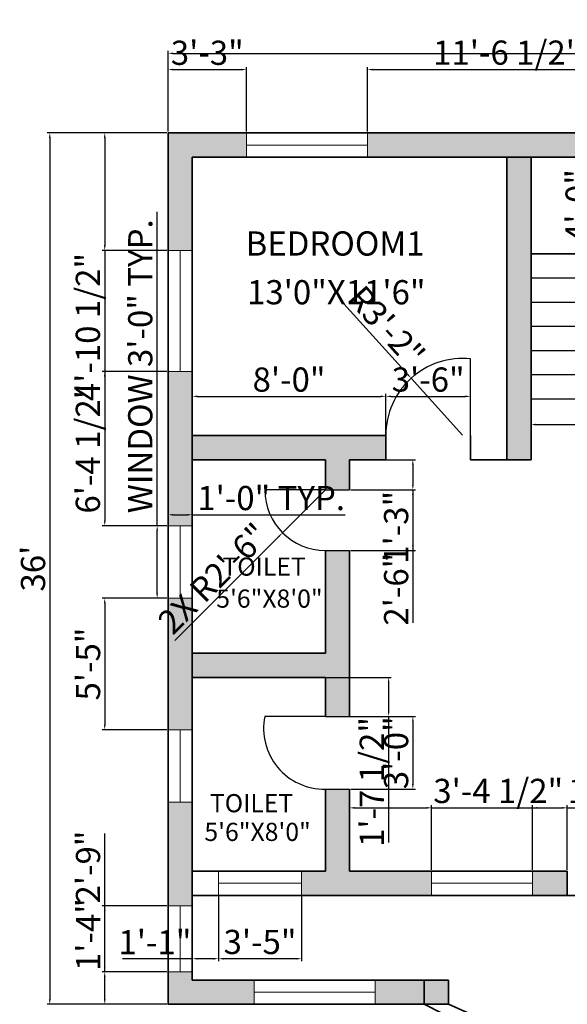
# Model space of a CAD drawing. Units: inches. Extents: x 1749 to 2426, y 1666 to 2412.
# Tile 2 of 3: x 1749 to 2021, y 1924 to 2412. Entities that reach past the tile are written whole.
import ezdxf

# ---------------------------------------------------------------- set-up
doc = ezdxf.new("R2010")
doc.units = ezdxf.units.IN
for name, color, linetype, lineweight in [('A-ANNO-DIMS', 2, 'Continuous', 18), ('A-AREA-IDEN', 4, 'Continuous', 18), ('A-DOOR', 6, 'Continuous', 25), ('A-FLOR-STRS', 7, 'Continuous', 25), ('A-GLAZ', 1, 'Continuous', 18), ('A-WALL', 2, 'Continuous', 35)]:
    doc.layers.add(name, color=color, linetype=linetype, lineweight=lineweight)
doc.layers.add('A-WALL-PATT', color=18, linetype='Continuous', lineweight=13, true_color=0x000000)
doc.styles.get("Standard").update_dxf_attribs({"font": 'arial.ttf'})
doc.dimstyles.new('ISO-25', dxfattribs={"dimtxt": 12, "dimasz": 2.5, "dimexe": 1.25, "dimexo": 0.625, "dimtad": 1, "dimdec": 0, "dimlunit": 3, "dimtxsty": 'Standard', "dimcen": 2.5, "dimadec": 0, "dimazin": 0, "dimtfac": 1, "dimtdec": 0, "dimtmove": 0, "dimatfit": 3, "dimfxl": 1, "dimarcsym": 0})

# ---------------------------------------------------------------- blocks, each defined once
blk = doc.blocks.new('*D1')
at = {"layer": 'A-ANNO-DIMS', "color": 0, "lineweight": -2, "transparency": 16777216}
for p, q in [((1822.59, 2356.85), (1822.59, 2396.9)), ((2374.59, 2356.85), (2374.59, 2396.9)), ((1825.09, 2395.65), (2372.09, 2395.65))]:
    blk.add_line(p, q, dxfattribs=at)
at = {"layer": 'A-ANNO-DIMS', "color": 0, "transparency": 16777216}
for points in [[(1825.09, 2396.07), (1825.09, 2395.23), (1822.59, 2395.65)], [(2372.09, 2396.07), (2372.09, 2395.23), (2374.59, 2395.65)]]:
    blk.add_solid(points, dxfattribs=at)
at = {"layer": 'Defpoints', "color": 0, "transparency": 16777216}
for p in [(2374.59, 2395.65), (1822.59, 2356.22), (2374.59, 2356.22)]:
    blk.add_point(p, dxfattribs=at)
at = {"layer": 'A-ANNO-DIMS', "color": 0, "transparency": 16777216, "insert": (2098.59, 2402.4), "char_height": 12, "attachment_point": 5}
blk.add_mtext("46'", dxfattribs=at)
blk = doc.blocks.new('*D2')
at = {"layer": 'A-ANNO-DIMS', "color": 0, "lineweight": -2, "transparency": 16777216}
for p, q in [((1821.97, 2356.22), (1762.68, 2356.22)), ((1763.93, 2353.72), (1763.93, 1926.72)), ((1821.97, 1924.22), (1762.68, 1924.22))]:
    blk.add_line(p, q, dxfattribs=at)
at = {"layer": 'A-ANNO-DIMS', "color": 0, "transparency": 16777216}
for points in [[(1763.52, 2353.72), (1764.35, 2353.72), (1763.93, 2356.22)], [(1763.52, 1926.72), (1764.35, 1926.72), (1763.93, 1924.22)]]:
    blk.add_solid(points, dxfattribs=at)
at = {"layer": 'Defpoints', "color": 0, "transparency": 16777216}
for p in [(1822.59, 2356.22), (1763.93, 1924.22), (1822.59, 1924.22)]:
    blk.add_point(p, dxfattribs=at)
at = {"layer": 'A-ANNO-DIMS', "color": 0, "transparency": 16777216, "insert": (1757.18, 2140.22), "char_height": 12, "attachment_point": 5, "rotation": 90}
blk.add_mtext("36'", dxfattribs=at)
blk = doc.blocks.new('WIN-60IN')
for p, q in [((12, 60), (0, 60)), ((6, 0), (6, 60)), ((6, 60), (12, 60)), ((0, 0), (12, 0))]:
    blk.add_line(p, q)
blk = doc.blocks.new('WIN-36IN')
for p, q in [((0, 36), (12, 36)), ((6, 36), (6, 0)), ((6, 0), (0, 0)), ((6, 0), (12, 0))]:
    blk.add_line(p, q)
blk = doc.blocks.new('WIN-50IN')
for p, q in [((0, 0), (0, 12)), ((50, 12), (50, 0)), ((50, 6), (0, 6)), ((0, 6), (0, 0))]:
    blk.add_line(p, q)
blk = doc.blocks.new('STAIR-FLIGHT-84IN')
for p, q in [((84, 72), (0, 72)), ((84, 60), (0, 60)), ((84, 48), (0, 48)), ((84, 36), (0, 36)), ((84, 24), (0, 24)), ((84, 12), (0, 12)), ((84, 0), (0, 0))]:
    blk.add_line(p, q)
blk = doc.blocks.new('*D9')
at = {"layer": 'A-ANNO-DIMS', "color": 0, "lineweight": -2, "transparency": 16777216}
for p, q in [((1817.19, 2161.49), (1817.19, 2317.09)), ((1821.97, 2161.49), (1815.94, 2161.49)), ((1817.19, 2127.99), (1817.19, 2158.99)), ((1821.97, 2125.49), (1815.94, 2125.49))]:
    blk.add_line(p, q, dxfattribs=at)
at = {"layer": 'A-ANNO-DIMS', "color": 0, "transparency": 16777216}
for points in [[(1816.77, 2158.99), (1817.61, 2158.99), (1817.19, 2161.49)], [(1816.77, 2127.99), (1817.61, 2127.99), (1817.19, 2125.49)]]:
    blk.add_solid(points, dxfattribs=at)
at = {"layer": 'Defpoints', "color": 0, "transparency": 16777216}
for p in [(1817.19, 2161.49), (1822.59, 2161.49), (1822.59, 2125.49)]:
    blk.add_point(p, dxfattribs=at)
at = {"layer": 'A-ANNO-DIMS', "color": 0, "transparency": 16777216, "insert": (1810.35, 2240.54), "char_height": 12, "attachment_point": 5, "rotation": 90}
blk.add_mtext('WINDOW 3\'-0" TYP.', dxfattribs=at)
blk = doc.blocks.new('*D10')
at = {"layer": 'A-ANNO-DIMS', "color": 0, "lineweight": -2, "transparency": 16777216}
for p, q in [((1822.59, 2162.12), (1822.59, 2168.14)), ((1834.59, 2162.12), (1834.59, 2168.14)), ((1825.09, 2166.89), (1832.09, 2166.89)), ((1834.59, 2166.89), (1910.36, 2166.89))]:
    blk.add_line(p, q, dxfattribs=at)
at = {"layer": 'A-ANNO-DIMS', "color": 0, "transparency": 16777216}
for points in [[(1825.09, 2167.31), (1825.09, 2166.48), (1822.59, 2166.89)], [(1832.09, 2167.31), (1832.09, 2166.48), (1834.59, 2166.89)]]:
    blk.add_solid(points, dxfattribs=at)
at = {"layer": 'Defpoints', "color": 0, "transparency": 16777216}
for p in [(1834.59, 2166.89), (1822.59, 2161.49), (1834.59, 2161.49)]:
    blk.add_point(p, dxfattribs=at)
at = {"layer": 'A-ANNO-DIMS', "color": 0, "transparency": 16777216, "insert": (1873.72, 2173.65), "char_height": 12, "attachment_point": 5}
blk.add_mtext('1\'-0" TYP.', dxfattribs=at)
blk = doc.blocks.new('*D13')
at = {"layer": 'A-ANNO-DIMS', "color": 0, "lineweight": -2, "transparency": 16777216}
for p, q in [((2002.59, 2223.6), (2002.59, 2210.37)), ((2086.59, 2223.6), (2086.59, 2210.37)), ((2005.09, 2211.62), (2084.09, 2211.62)), ((2086.59, 2211.62), (2281.72, 2211.62))]:
    blk.add_line(p, q, dxfattribs=at)
at = {"layer": 'A-ANNO-DIMS', "color": 0, "transparency": 16777216}
for points in [[(2005.09, 2212.04), (2005.09, 2211.2), (2002.59, 2211.62)], [(2084.09, 2212.04), (2084.09, 2211.2), (2086.59, 2211.62)]]:
    blk.add_solid(points, dxfattribs=at)
at = {"layer": 'Defpoints', "color": 0, "transparency": 16777216}
for p in [(2002.59, 2224.22), (2086.59, 2224.22), (2086.59, 2211.62)]:
    blk.add_point(p, dxfattribs=at)
at = {"layer": 'A-ANNO-DIMS', "color": 0, "transparency": 16777216, "insert": (2185.41, 2218.45), "char_height": 12, "attachment_point": 5}
blk.add_mtext('STAIR FLIGHT 7\'-0" TYP.', dxfattribs=at)
blk = doc.blocks.new('*D15')
at = {"layer": 'A-ANNO-DIMS', "color": 0, "lineweight": -2, "transparency": 16777216}
for p, q in [((1822.59, 2356.85), (1822.59, 2388.87)), ((1825.09, 2387.62), (1858.99, 2387.62)), ((1861.49, 2356.85), (1861.49, 2388.87))]:
    blk.add_line(p, q, dxfattribs=at)
at = {"layer": 'A-ANNO-DIMS', "color": 0, "transparency": 16777216}
for points in [[(1825.09, 2388.04), (1825.09, 2387.2), (1822.59, 2387.62)], [(1858.99, 2388.04), (1858.99, 2387.2), (1861.49, 2387.62)]]:
    blk.add_solid(points, dxfattribs=at)
at = {"layer": 'Defpoints', "color": 0, "transparency": 16777216}
for p in [(1861.49, 2387.62), (1822.59, 2356.22), (1861.49, 2356.22)]:
    blk.add_point(p, dxfattribs=at)
at = {"layer": 'A-ANNO-DIMS', "color": 0, "transparency": 16777216, "insert": (1842.04, 2394.38), "char_height": 12, "attachment_point": 5}
blk.add_mtext('3\'-3"', dxfattribs=at)
blk = doc.blocks.new('*D16')
at = {"layer": 'A-ANNO-DIMS', "color": 0, "lineweight": -2, "transparency": 16777216}
for p, q in [((1921.49, 2356.85), (1921.49, 2388.87)), ((1923.99, 2387.62), (2057.63, 2387.62)), ((2060.13, 2356.85), (2060.13, 2388.87))]:
    blk.add_line(p, q, dxfattribs=at)
at = {"layer": 'A-ANNO-DIMS', "color": 0, "transparency": 16777216}
for points in [[(1923.99, 2388.04), (1923.99, 2387.2), (1921.49, 2387.62)], [(2057.63, 2388.04), (2057.63, 2387.2), (2060.13, 2387.62)]]:
    blk.add_solid(points, dxfattribs=at)
at = {"layer": 'Defpoints', "color": 0, "transparency": 16777216}
for p in [(2060.13, 2387.62), (1921.49, 2356.22), (2060.13, 2356.22)]:
    blk.add_point(p, dxfattribs=at)
at = {"layer": 'A-ANNO-DIMS', "color": 0, "transparency": 16777216, "insert": (1990.81, 2394.45), "char_height": 12, "attachment_point": 5}
blk.add_mtext('11\'-6 1/2"', dxfattribs=at)
blk = doc.blocks.new('*D19')
at = {"layer": 'A-ANNO-DIMS', "color": 0, "lineweight": -2, "transparency": 16777216}
for p, q in [((1821.97, 2356.22), (1789.94, 2356.22)), ((1791.19, 2353.72), (1791.19, 2300.45)), ((1821.97, 2297.95), (1789.94, 2297.95)), ((1791.19, 2297.95), (1791.19, 2224.53))]:
    blk.add_line(p, q, dxfattribs=at)
at = {"layer": 'A-ANNO-DIMS', "color": 0, "transparency": 16777216}
for points in [[(1790.77, 2353.72), (1791.61, 2353.72), (1791.19, 2356.22)], [(1790.77, 2300.45), (1791.61, 2300.45), (1791.19, 2297.95)]]:
    blk.add_solid(points, dxfattribs=at)
at = {"layer": 'Defpoints', "color": 0, "transparency": 16777216}
for p in [(1822.59, 2356.22), (1791.19, 2297.95), (1822.59, 2297.95)]:
    blk.add_point(p, dxfattribs=at)
at = {"layer": 'A-ANNO-DIMS', "color": 0, "transparency": 16777216, "insert": (1784.36, 2259.99), "char_height": 12, "attachment_point": 5, "rotation": 90}
blk.add_mtext('4\'-10 1/2"', dxfattribs=at)
blk = doc.blocks.new('*D20')
at = {"layer": 'A-ANNO-DIMS', "color": 0, "lineweight": -2, "transparency": 16777216}
for p, q in [((1821.97, 2237.95), (1789.94, 2237.95)), ((1791.19, 2235.45), (1791.19, 2163.99)), ((1821.97, 2161.49), (1789.94, 2161.49))]:
    blk.add_line(p, q, dxfattribs=at)
at = {"layer": 'A-ANNO-DIMS', "color": 0, "transparency": 16777216}
for points in [[(1790.77, 2235.45), (1791.61, 2235.45), (1791.19, 2237.95)], [(1790.77, 2163.99), (1791.61, 2163.99), (1791.19, 2161.49)]]:
    blk.add_solid(points, dxfattribs=at)
at = {"layer": 'Defpoints', "color": 0, "transparency": 16777216}
for p in [(1822.59, 2237.95), (1791.19, 2161.49), (1822.59, 2161.49)]:
    blk.add_point(p, dxfattribs=at)
at = {"layer": 'A-ANNO-DIMS', "color": 0, "transparency": 16777216, "insert": (1784.36, 2199.72), "char_height": 12, "attachment_point": 5, "rotation": 90}
blk.add_mtext('6\'-4 1/2"', dxfattribs=at)
blk = doc.blocks.new('*D21')
at = {"layer": 'A-ANNO-DIMS', "color": 0, "lineweight": -2, "transparency": 16777216}
for p, q in [((1821.97, 2125.49), (1789.94, 2125.49)), ((1791.19, 2122.99), (1791.19, 2062.85)), ((1821.97, 2060.35), (1789.94, 2060.35))]:
    blk.add_line(p, q, dxfattribs=at)
at = {"layer": 'A-ANNO-DIMS', "color": 0, "transparency": 16777216}
for points in [[(1790.77, 2122.99), (1791.61, 2122.99), (1791.19, 2125.49)], [(1790.77, 2062.85), (1791.61, 2062.85), (1791.19, 2060.35)]]:
    blk.add_solid(points, dxfattribs=at)
at = {"layer": 'Defpoints', "color": 0, "transparency": 16777216}
for p in [(1822.59, 2125.49), (1791.19, 2060.35), (1822.59, 2060.35)]:
    blk.add_point(p, dxfattribs=at)
at = {"layer": 'A-ANNO-DIMS', "color": 0, "transparency": 16777216, "insert": (1784.46, 2092.92), "char_height": 12, "attachment_point": 5, "rotation": 90}
blk.add_mtext('5\'-5"', dxfattribs=at)
blk = doc.blocks.new('*D29')
at = {"layer": 'A-ANNO-DIMS', "color": 0, "lineweight": -2, "transparency": 16777216}
for p, q in [((1834.59, 2194.85), (1834.59, 2226.87)), ((1930.59, 2194.85), (1930.59, 2226.87)), ((1837.09, 2225.62), (1928.09, 2225.62))]:
    blk.add_line(p, q, dxfattribs=at)
at = {"layer": 'A-ANNO-DIMS', "color": 0, "transparency": 16777216}
for points in [[(1837.09, 2226.04), (1837.09, 2225.2), (1834.59, 2225.62)], [(1928.09, 2226.04), (1928.09, 2225.2), (1930.59, 2225.62)]]:
    blk.add_solid(points, dxfattribs=at)
at = {"layer": 'Defpoints', "color": 0, "transparency": 16777216}
for p in [(1930.59, 2225.62), (1834.59, 2194.22), (1930.59, 2194.22)]:
    blk.add_point(p, dxfattribs=at)
at = {"layer": 'A-ANNO-DIMS', "color": 0, "transparency": 16777216, "insert": (1882.59, 2232.37), "char_height": 12, "attachment_point": 5}
blk.add_mtext('8\'-0"', dxfattribs=at)
blk = doc.blocks.new('*D30')
at = {"layer": 'A-ANNO-DIMS', "color": 0, "lineweight": -2, "transparency": 16777216}
for p, q in [((1930.59, 2194.85), (1930.59, 2226.87)), ((1972.59, 2194.85), (1972.59, 2226.87)), ((1933.09, 2225.62), (1970.09, 2225.62))]:
    blk.add_line(p, q, dxfattribs=at)
at = {"layer": 'A-ANNO-DIMS', "color": 0, "transparency": 16777216}
for points in [[(1933.09, 2226.04), (1933.09, 2225.2), (1930.59, 2225.62)], [(1970.09, 2226.04), (1970.09, 2225.2), (1972.59, 2225.62)]]:
    blk.add_solid(points, dxfattribs=at)
at = {"layer": 'Defpoints', "color": 0, "transparency": 16777216}
for p in [(1972.59, 2225.62), (1930.59, 2194.22), (1972.59, 2194.22)]:
    blk.add_point(p, dxfattribs=at)
at = {"layer": 'A-ANNO-DIMS', "color": 0, "transparency": 16777216, "insert": (1951.59, 2232.38), "char_height": 12, "attachment_point": 5}
blk.add_mtext('3\'-6"', dxfattribs=at)
blk = doc.blocks.new('*D33')
at = {"layer": 'A-ANNO-DIMS', "color": 0, "lineweight": -2, "transparency": 16777216}
for p, q in [((2003.22, 2344.22), (2035.24, 2344.22)), ((2033.99, 2341.72), (2033.99, 2298.72)), ((2003.22, 2296.22), (2035.24, 2296.22))]:
    blk.add_line(p, q, dxfattribs=at)
at = {"layer": 'A-ANNO-DIMS', "color": 0, "transparency": 16777216}
for points in [[(2033.57, 2341.72), (2034.41, 2341.72), (2033.99, 2344.22)], [(2033.57, 2298.72), (2034.41, 2298.72), (2033.99, 2296.22)]]:
    blk.add_solid(points, dxfattribs=at)
at = {"layer": 'Defpoints', "color": 0, "transparency": 16777216}
for p in [(2002.59, 2344.22), (2002.59, 2296.22), (2033.99, 2296.22)]:
    blk.add_point(p, dxfattribs=at)
at = {"layer": 'A-ANNO-DIMS', "color": 0, "transparency": 16777216, "insert": (2027.24, 2320.22), "char_height": 12, "attachment_point": 5, "rotation": 90}
blk.add_mtext('4\'-0"', dxfattribs=at)
blk = doc.blocks.new('*D40')
at = {"layer": 'A-ANNO-DIMS', "color": 0, "lineweight": -2, "transparency": 16777216}
for p, q in [((1791.19, 1973.11), (1791.19, 2008.96)), ((1821.97, 1973.11), (1789.94, 1973.11)), ((1791.19, 1942.77), (1791.19, 1970.61)), ((1821.97, 1940.27), (1789.94, 1940.27))]:
    blk.add_line(p, q, dxfattribs=at)
at = {"layer": 'A-ANNO-DIMS', "color": 0, "transparency": 16777216}
for points in [[(1790.77, 1970.61), (1791.61, 1970.61), (1791.19, 1973.11)], [(1790.77, 1942.77), (1791.61, 1942.77), (1791.19, 1940.27)]]:
    blk.add_solid(points, dxfattribs=at)
at = {"layer": 'Defpoints', "color": 0, "transparency": 16777216}
for p in [(1791.19, 1973.11), (1822.59, 1973.11), (1822.59, 1940.27)]:
    blk.add_point(p, dxfattribs=at)
at = {"layer": 'A-ANNO-DIMS', "color": 0, "transparency": 16777216, "insert": (1784.44, 1992.28), "char_height": 12, "attachment_point": 5, "rotation": 90}
blk.add_mtext('2\'-9"', dxfattribs=at)
blk = doc.blocks.new('*D41')
at = {"layer": 'A-ANNO-DIMS', "color": 0, "lineweight": -2, "transparency": 16777216}
for p, q in [((1791.19, 1940.27), (1791.19, 1974.79)), ((1821.97, 1940.27), (1789.94, 1940.27)), ((1791.19, 1926.72), (1791.19, 1937.77)), ((1821.97, 1924.22), (1789.94, 1924.22))]:
    blk.add_line(p, q, dxfattribs=at)
at = {"layer": 'A-ANNO-DIMS', "color": 0, "transparency": 16777216}
for points in [[(1790.77, 1937.77), (1791.61, 1937.77), (1791.19, 1940.27)], [(1790.77, 1926.72), (1791.61, 1926.72), (1791.19, 1924.22)]]:
    blk.add_solid(points, dxfattribs=at)
at = {"layer": 'Defpoints', "color": 0, "transparency": 16777216}
for p in [(1791.19, 1940.27), (1822.59, 1940.27), (1822.59, 1924.22)]:
    blk.add_point(p, dxfattribs=at)
at = {"layer": 'A-ANNO-DIMS', "color": 0, "transparency": 16777216, "insert": (1784.54, 1958.78), "char_height": 12, "attachment_point": 5, "rotation": 90}
blk.add_mtext('1\'-4"', dxfattribs=at)
blk = doc.blocks.new('*D46')
at = {"layer": 'A-ANNO-DIMS', "color": 0, "lineweight": -2, "transparency": 16777216}
for p, q in [((1847.61, 1977.6), (1847.61, 1945.57)), ((1888.8, 1977.6), (1888.8, 1945.57)), ((1886.3, 1946.82), (1850.11, 1946.82))]:
    blk.add_line(p, q, dxfattribs=at)
at = {"layer": 'A-ANNO-DIMS', "color": 0, "transparency": 16777216}
for points in [[(1850.11, 1947.24), (1850.11, 1946.4), (1847.61, 1946.82)], [(1886.3, 1947.24), (1886.3, 1946.4), (1888.8, 1946.82)]]:
    blk.add_solid(points, dxfattribs=at)
at = {"layer": 'Defpoints', "color": 0, "transparency": 16777216}
for p in [(1847.61, 1978.22), (1888.8, 1978.22), (1847.61, 1946.82)]:
    blk.add_point(p, dxfattribs=at)
at = {"layer": 'A-ANNO-DIMS', "color": 0, "transparency": 16777216, "insert": (1868.2, 1953.58), "char_height": 12, "attachment_point": 5}
blk.add_mtext('3\'-5"', dxfattribs=at)
blk = doc.blocks.new('*D47')
at = {"layer": 'A-ANNO-DIMS', "color": 0, "lineweight": -2, "transparency": 16777216}
for p, q in [((1834.59, 1977.6), (1834.59, 1945.57)), ((1847.61, 1977.6), (1847.61, 1945.57)), ((1834.59, 1946.82), (1800.07, 1946.82)), ((1845.11, 1946.82), (1837.09, 1946.82))]:
    blk.add_line(p, q, dxfattribs=at)
at = {"layer": 'A-ANNO-DIMS', "color": 0, "transparency": 16777216}
for points in [[(1837.09, 1947.24), (1837.09, 1946.4), (1834.59, 1946.82)], [(1845.11, 1947.24), (1845.11, 1946.4), (1847.61, 1946.82)]]:
    blk.add_solid(points, dxfattribs=at)
at = {"layer": 'Defpoints', "color": 0, "transparency": 16777216}
for p in [(1834.59, 1978.22), (1847.61, 1978.22), (1834.59, 1946.82)]:
    blk.add_point(p, dxfattribs=at)
at = {"layer": 'A-ANNO-DIMS', "color": 0, "transparency": 16777216, "insert": (1816.08, 1953.47), "char_height": 12, "attachment_point": 5}
blk.add_mtext('1\'-1"', dxfattribs=at)
blk = doc.blocks.new('*D48')
at = {"layer": 'A-ANNO-DIMS', "color": 0, "lineweight": -2, "transparency": 16777216}
for p, q in [((1912.59, 1990.85), (1912.59, 2022.87)), ((1915.09, 2021.62), (1950.79, 2021.62)), ((1953.29, 1990.85), (1953.29, 2022.87)), ((1953.29, 2021.62), (2016.89, 2021.62))]:
    blk.add_line(p, q, dxfattribs=at)
at = {"layer": 'A-ANNO-DIMS', "color": 0, "transparency": 16777216}
for points in [[(1915.09, 2022.04), (1915.09, 2021.2), (1912.59, 2021.62)], [(1950.79, 2022.04), (1950.79, 2021.2), (1953.29, 2021.62)]]:
    blk.add_solid(points, dxfattribs=at)
at = {"layer": 'Defpoints', "color": 0, "transparency": 16777216}
for p in [(1953.29, 2021.62), (1912.59, 1990.22), (1953.29, 1990.22)]:
    blk.add_point(p, dxfattribs=at)
at = {"layer": 'A-ANNO-DIMS', "color": 0, "transparency": 16777216, "insert": (1986.34, 2028.45), "char_height": 12, "attachment_point": 5}
blk.add_mtext('3\'-4 1/2"', dxfattribs=at)
blk = doc.blocks.new('*D49')
at = {"layer": 'A-ANNO-DIMS', "color": 0, "lineweight": -2, "transparency": 16777216}
for p, q in [((2003.29, 1990.85), (2003.29, 2022.87)), ((2005.79, 2021.62), (2018.09, 2021.62)), ((2020.59, 1990.85), (2020.59, 2022.87)), ((2020.59, 2021.62), (2083.07, 2021.62))]:
    blk.add_line(p, q, dxfattribs=at)
at = {"layer": 'A-ANNO-DIMS', "color": 0, "transparency": 16777216}
for points in [[(2005.79, 2022.04), (2005.79, 2021.2), (2003.29, 2021.62)], [(2018.09, 2022.04), (2018.09, 2021.2), (2020.59, 2021.62)]]:
    blk.add_solid(points, dxfattribs=at)
at = {"layer": 'Defpoints', "color": 0, "transparency": 16777216}
for p in [(2020.59, 2021.62), (2003.29, 1990.22), (2020.59, 1990.22)]:
    blk.add_point(p, dxfattribs=at)
at = {"layer": 'A-ANNO-DIMS', "color": 0, "transparency": 16777216, "insert": (2053.08, 2028.45), "char_height": 12, "attachment_point": 5}
blk.add_mtext('1\'-5 1/2"', dxfattribs=at)
blk = doc.blocks.new('*D52')
at = {"layer": 'A-ANNO-DIMS', "color": 0, "lineweight": -2, "transparency": 16777216}
for p, q in [((1913.22, 2194.22), (1945.24, 2194.22)), ((1943.99, 2191.72), (1943.99, 2181.72)), ((1913.22, 2179.22), (1945.24, 2179.22)), ((1943.99, 2179.22), (1943.99, 2144.7))]:
    blk.add_line(p, q, dxfattribs=at)
at = {"layer": 'A-ANNO-DIMS', "color": 0, "transparency": 16777216}
for points in [[(1943.57, 2191.72), (1944.41, 2191.72), (1943.99, 2194.22)], [(1943.57, 2181.72), (1944.41, 2181.72), (1943.99, 2179.22)]]:
    blk.add_solid(points, dxfattribs=at)
at = {"layer": 'Defpoints', "color": 0, "transparency": 16777216}
for p in [(1912.59, 2194.22), (1912.59, 2179.22), (1943.99, 2179.22)]:
    blk.add_point(p, dxfattribs=at)
at = {"layer": 'A-ANNO-DIMS', "color": 0, "transparency": 16777216, "insert": (1937.24, 2160.71), "char_height": 12, "attachment_point": 5, "rotation": 90}
blk.add_mtext('1\'-3"', dxfattribs=at)
blk = doc.blocks.new('*D53')
at = {"layer": 'A-ANNO-DIMS', "color": 0, "lineweight": -2, "transparency": 16777216}
for p, q in [((1913.22, 2179.22), (1945.24, 2179.22)), ((1943.99, 2176.72), (1943.99, 2151.72)), ((1913.22, 2149.22), (1945.24, 2149.22)), ((1943.99, 2149.22), (1943.99, 2113.37))]:
    blk.add_line(p, q, dxfattribs=at)
at = {"layer": 'A-ANNO-DIMS', "color": 0, "transparency": 16777216}
for points in [[(1943.57, 2176.72), (1944.41, 2176.72), (1943.99, 2179.22)], [(1943.57, 2151.72), (1944.41, 2151.72), (1943.99, 2149.22)]]:
    blk.add_solid(points, dxfattribs=at)
at = {"layer": 'Defpoints', "color": 0, "transparency": 16777216}
for p in [(1912.59, 2179.22), (1912.59, 2149.22), (1943.99, 2149.22)]:
    blk.add_point(p, dxfattribs=at)
at = {"layer": 'A-ANNO-DIMS', "color": 0, "transparency": 16777216, "insert": (1937.24, 2130.04), "char_height": 12, "attachment_point": 5, "rotation": 90}
blk.add_mtext('2\'-6"', dxfattribs=at)
blk = doc.blocks.new('*D54')
at = {"layer": 'A-ANNO-DIMS', "color": 0, "lineweight": -2, "transparency": 16777216}
for p, q in [((1901.22, 2086.22), (1933.24, 2086.22)), ((1931.99, 2083.72), (1931.99, 2069.44)), ((1901.22, 2066.94), (1933.24, 2066.94)), ((1931.99, 2066.94), (1931.99, 2004.46))]:
    blk.add_line(p, q, dxfattribs=at)
at = {"layer": 'A-ANNO-DIMS', "color": 0, "transparency": 16777216}
for points in [[(1931.57, 2083.72), (1932.41, 2083.72), (1931.99, 2086.22)], [(1931.57, 2069.44), (1932.41, 2069.44), (1931.99, 2066.94)]]:
    blk.add_solid(points, dxfattribs=at)
at = {"layer": 'Defpoints', "color": 0, "transparency": 16777216}
for p in [(1900.59, 2086.22), (1900.59, 2066.94), (1931.99, 2066.94)]:
    blk.add_point(p, dxfattribs=at)
at = {"layer": 'A-ANNO-DIMS', "color": 0, "transparency": 16777216, "insert": (1925.16, 2034.45), "char_height": 12, "attachment_point": 5, "rotation": 90}
blk.add_mtext('1\'-7 1/2"', dxfattribs=at)
blk = doc.blocks.new('*D55')
at = {"layer": 'A-ANNO-DIMS', "color": 0, "lineweight": -2, "transparency": 16777216}
for p, q in [((1913.22, 2066.94), (1945.24, 2066.94)), ((1943.99, 2064.44), (1943.99, 2033.44)), ((1913.22, 2030.94), (1945.24, 2030.94))]:
    blk.add_line(p, q, dxfattribs=at)
at = {"layer": 'A-ANNO-DIMS', "color": 0, "transparency": 16777216}
for points in [[(1943.57, 2064.44), (1944.41, 2064.44), (1943.99, 2066.94)], [(1943.57, 2033.44), (1944.41, 2033.44), (1943.99, 2030.94)]]:
    blk.add_solid(points, dxfattribs=at)
at = {"layer": 'Defpoints', "color": 0, "transparency": 16777216}
for p in [(1912.59, 2066.94), (1912.59, 2030.94), (1943.99, 2030.94)]:
    blk.add_point(p, dxfattribs=at)
at = {"layer": 'A-ANNO-DIMS', "color": 0, "transparency": 16777216, "insert": (1937.24, 2048.94), "char_height": 12, "attachment_point": 5, "rotation": 90}
blk.add_mtext('3\'-0"', dxfattribs=at)
blk = doc.blocks.new('*D59')
at = {"layer": 'A-ANNO-DIMS', "color": 0, "lineweight": -2, "transparency": 16777216}
for p, q in [((1909.8, 2271.41), (1941.42, 2236.46)), ((1968.59, 2206.43), (1943.1, 2234.61))]:
    blk.add_line(p, q, dxfattribs=at)
at = {"layer": 'A-ANNO-DIMS', "color": 0, "transparency": 16777216}
blk.add_solid([(1941.73, 2236.74), (1941.11, 2236.18), (1943.1, 2234.61)], dxfattribs=at)
at = {"layer": 'Defpoints', "color": 0, "transparency": 16777216}
for p in [(1943.1, 2234.61), (1968.59, 2206.43)]:
    blk.add_point(p, dxfattribs=at)
at = {"layer": 'A-ANNO-DIMS', "color": 0, "transparency": 16777216, "insert": (1929.78, 2259.4), "char_height": 12, "attachment_point": 5, "rotation": 312.1383}
blk.add_mtext('R3\'-2"', dxfattribs=at)
blk = doc.blocks.new('*D60')
at = {"layer": 'A-ANNO-DIMS', "color": 0, "lineweight": -2, "transparency": 16777216}
for p, q in [((1900.59, 2179.22), (1879.38, 2158.01)), ((1825.9, 2104.54), (1877.61, 2156.24))]:
    blk.add_line(p, q, dxfattribs=at)
at = {"layer": 'A-ANNO-DIMS', "color": 0, "transparency": 16777216}
blk.add_solid([(1877.32, 2156.53), (1877.9, 2155.95), (1879.38, 2158.01)], dxfattribs=at)
at = {"layer": 'Defpoints', "color": 0, "transparency": 16777216}
for p in [(1900.59, 2179.22), (1879.38, 2158.01)]:
    blk.add_point(p, dxfattribs=at)
at = {"layer": 'A-ANNO-DIMS', "color": 0, "transparency": 16777216, "insert": (1846.1, 2134.28), "char_height": 12, "attachment_point": 5, "rotation": 44.9992}
blk.add_mtext('2X R2\'-6"', dxfattribs=at)

msp = doc.modelspace()

# ---------------------------------------------------------------- hatches: boundary and pattern name
at = {"layer": 'A-WALL-PATT'}
h = msp.add_hatch(color=256, dxfattribs=at)
h.dxf.hatch_style = 1
h.paths.add_polyline_path([(1834.59, 2344.22), (1861.49, 2344.22), (1861.49, 2356.22), (1822.59, 2356.22), (1822.59, 2297.95), (1834.59, 2297.95)])
h = msp.add_hatch(color=256, dxfattribs=at)
h.dxf.hatch_style = 1
h.paths.add_polyline_path([(2060.13, 2344.22), (2060.13, 2356.22), (1921.49, 2356.22), (1921.49, 2344.22)])
h = msp.add_hatch(color=256, dxfattribs=at)
h.dxf.hatch_style = 1
h.paths.add_polyline_path([(2002.59, 2344.22), (1990.59, 2344.22), (1990.59, 2194.22), (2002.59, 2194.22)])
h = msp.add_hatch(color=256, dxfattribs=at)
h.dxf.hatch_style = 1
h.paths.add_polyline_path([(1834.59, 2237.95), (1822.59, 2237.95), (1822.59, 2161.49), (1834.59, 2161.49)])
h = msp.add_hatch(color=256, dxfattribs=at)
h.dxf.hatch_style = 1
h.paths.add_polyline_path([(1834.59, 2206.22), (1834.59, 2194.22), (1900.59, 2194.22), (1900.59, 2179.22), (1912.59, 2179.22), (1912.59, 2194.22), (1930.59, 2194.22), (1930.59, 2206.22)])
h = msp.add_hatch(color=256, dxfattribs=at)
h.dxf.hatch_style = 1
h.paths.add_polyline_path([(1900.59, 2098.22), (1834.59, 2098.22), (1834.59, 2086.22), (1900.59, 2086.22), (1900.59, 2066.94), (1912.59, 2066.94), (1912.59, 2149.22), (1900.59, 2149.22)])
h = msp.add_hatch(color=256, dxfattribs=at)
h.dxf.hatch_style = 1
h.paths.add_polyline_path([(1834.59, 2125.49), (1828.59, 2125.49), (1822.59, 2125.49), (1822.59, 2060.35), (1834.59, 2060.35)])
h = msp.add_hatch(color=256, dxfattribs=at)
h.dxf.hatch_style = 1
h.paths.add_polyline_path([(1912.59, 1990.22), (1912.59, 2030.94), (1900.59, 2030.94), (1900.59, 1990.22), (1888.8, 1990.22), (1888.8, 1978.22), (1953.29, 1978.22), (1953.29, 1990.22)])
h = msp.add_hatch(color=256, dxfattribs=at)
h.dxf.hatch_style = 1
h.paths.add_polyline_path([(1822.59, 1973.11), (1834.59, 1973.11), (1834.59, 2024.35), (1828.59, 2024.35), (1822.59, 2024.35)])
h = msp.add_hatch(color=256, dxfattribs=at)
h.dxf.hatch_style = 1
h.paths.add_polyline_path([(2020.59, 1978.22), (2020.59, 1990.22), (2003.29, 1990.22), (2003.29, 1978.22)])
h = msp.add_hatch(color=256, dxfattribs=at)
h.dxf.hatch_style = 1
h.paths.add_polyline_path([(1865.37, 1924.22), (1865.37, 1936.22), (1834.59, 1936.22), (1834.59, 1940.27), (1822.59, 1940.27), (1822.59, 1924.22)])
h = msp.add_hatch(color=256, dxfattribs=at)
h.dxf.hatch_style = 1
h.paths.add_polyline_path([(1949.59, 1936.22), (1925.37, 1936.22), (1925.37, 1924.22), (1949.59, 1924.22)])
h = msp.add_hatch(color=256, dxfattribs=at)
h.dxf.hatch_style = 1
h.paths.add_polyline_path([(1961.59, 1936.22), (1949.59, 1936.22), (1949.59, 1924.22), (1961.59, 1924.22)])

# ---------------------------------------------------------------- linework, layer by layer
at = {"layer": 'A-DOOR'}
for p, q in [((1972.59, 2194.22), (1972.59, 2244.22)), ((1900.59, 2179.22), (1870.59, 2179.22)), ((1900.59, 2179.22), (1912.59, 2179.22)), ((1900.59, 2149.22), (1912.59, 2149.22)), ((1900.59, 2066.94), (1912.59, 2066.94)), ((1900.59, 2030.94), (1912.59, 2030.94))]:
    msp.add_line(p, q, dxfattribs=at)
msp.add_lwpolyline([(1900.59, 2066.94), (1870.59, 2066.94)], dxfattribs=at)
for centre, radius, start, end in [((1968.59, 2206.43), 38, 83.9568, 180.3184), ((1900.59, 2179.22), 30, 180, 270), ((1899.98, 2060.93), 30, 168.4511, 271.1601)]:
    msp.add_arc(centre, radius, start, end, dxfattribs=at)
at = {"layer": 'A-GLAZ'}
for p, q in [((1847.61, 1990.22), (1847.61, 1978.22)), ((1888.8, 1978.22), (1888.8, 1990.22)), ((1888.8, 1984.22), (1847.61, 1984.22)), ((1834.59, 1973.11), (1822.59, 1973.11)), ((1828.59, 1973.11), (1828.59, 1940.27)), ((1834.59, 1940.27), (1822.59, 1940.27))]:
    msp.add_line(p, q, dxfattribs=at)
at = {"layer": 'A-WALL'}
for p, q in [((1834.59, 2344.22), (2362.59, 2344.22)), ((1834.59, 1936.22), (1834.59, 2344.22)), ((1990.59, 2194.22), (1990.59, 2344.22)), ((2002.59, 2194.22), (2002.59, 2344.22)), ((1834.59, 2206.22), (1930.59, 2206.22)), ((1930.59, 2194.22), (1930.59, 2206.22)), ((1972.59, 2194.22), (1972.59, 2206.22)), ((1834.59, 2194.22), (1900.59, 2194.22)), ((1900.59, 2179.22), (1900.59, 2194.22)), ((1912.59, 2194.22), (1930.59, 2194.22)), ((1912.59, 2179.22), (1912.59, 2194.22)), ((1972.59, 2194.22), (2002.59, 2194.22)), ((1900.59, 2098.22), (1900.59, 2149.22)), ((1912.59, 2066.94), (1912.59, 2149.22)), ((1834.59, 2098.22), (1900.59, 2098.22)), ((1834.59, 2086.22), (1900.59, 2086.22)), ((1900.59, 2066.94), (1900.59, 2086.22)), ((1900.59, 1990.22), (1900.59, 2030.94)), ((1912.59, 1990.22), (1912.59, 2030.94)), ((1834.59, 1990.22), (1900.59, 1990.22)), ((1912.59, 1990.22), (2020.59, 1990.22)), ((2020.59, 1990.22), (2020.59, 1978.22)), ((1834.59, 1978.22), (2362.59, 1978.22)), ((1961.59, 1936.22), (1834.59, 1936.22)), ((1949.59, 1936.22), (1949.59, 1924.22)), ((1961.59, 1936.22), (1961.59, 1924.22))]:
    msp.add_line(p, q, dxfattribs=at)
msp.add_lwpolyline([(1961.59, 1924.22), (1822.59, 1924.22), (1822.59, 2356.22), (2374.59, 2356.22), (2374.59, 1924.22), (2235.59, 1924.22)], dxfattribs=at)
for centre, radius, start, end in [((2098.59, 2211.93), 324, 242.6209, 297.3791), ((2098.59, 2231.02), 336, 245.9372, 294.0628)]:
    msp.add_arc(centre, radius, start, end, dxfattribs=at)

# ---------------------------------------------------------------- block references
at = {"layer": 'A-FLOR-STRS'}
msp.add_blockref('STAIR-FLIGHT-84IN', (2002.59, 2224.22), dxfattribs=at)
at = {"layer": 'A-GLAZ', "extrusion": (0, 0, -1), "zscale": -1}
for p, rotation in [((-1861.49, 2344.22), 89.99999999999896), ((-1925.37, 1936.22), 270.0000000000003)]:
    msp.add_blockref('WIN-60IN', p, dxfattribs=dict(at, rotation=rotation))
at = {"layer": 'A-GLAZ'}
for name, p in [('WIN-60IN', (1822.59, 2237.95)), ('WIN-36IN', (1822.59, 2125.49)), ('WIN-36IN', (1822.59, 2024.35)), ('WIN-50IN', (1953.29, 1978.22))]:
    msp.add_blockref(name, p, dxfattribs=at)

# ---------------------------------------------------------------- texts
at = {"layer": 'A-AREA-IDEN'}
for tag, p, height in [('BEDROOM1', (1861.03, 2295.39), 12), ('13\'0"X11\'6"', (1861.77, 2271.23), 12), ('TOILET', (1849.56, 2136.72), 9), ('5\'6"X8\'0"', (1846.49, 2120.86), 9), ('TOILET', (1843.34, 2019.43), 9), ('5\'6"X8\'0"', (1840.61, 2005.2), 9)]:
    msp.add_attdef(tag, p, '', height=height, dxfattribs=at)

# ---------------------------------------------------------------- dimensions: what is measured, and where the dimension line sits
at = {"layer": 'A-ANNO-DIMS'}
for base, p1, p2, override, picture, middle in [((2060.13, 2387.62), (1921.49, 2356.22), (2060.13, 2356.22), {"dimdec": 1, "dimlfac": 1, "dimrnd": 0, "dimzin": 1, "dimdsep": 46, "dimlunit": 4, "dimfrac": 2}, '*D16', (1990.81, 2394.45)), ((2374.59, 2395.65), (1822.59, 2356.22), (2374.59, 2356.22), {"dimclrd": 0, "dimclre": 0, "dimclrt": 0}, '*D1', (2098.59, 2402.4)), ((1861.49, 2387.62), (1822.59, 2356.22), (1861.49, 2356.22), {"dimdec": 1, "dimlfac": 1, "dimrnd": 0, "dimzin": 1, "dimdsep": 46, "dimlunit": 4, "dimfrac": 2}, '*D15', (1842.04, 2394.38)), ((1930.59, 2225.62), (1834.59, 2194.22), (1930.59, 2194.22), {"dimdec": 1, "dimlfac": 1, "dimrnd": 0, "dimzin": 1, "dimdsep": 46, "dimlunit": 4, "dimfrac": 2}, '*D29', (1882.59, 2232.37)), ((1972.59, 2225.62), (1930.59, 2194.22), (1972.59, 2194.22), {"dimdec": 1, "dimlfac": 1, "dimrnd": 0, "dimzin": 1, "dimdsep": 46, "dimlunit": 4, "dimfrac": 2}, '*D30', (1951.59, 2232.38)), ((1953.29, 2021.62), (1912.59, 1990.22), (1953.29, 1990.22), {"dimdec": 1, "dimlfac": 1, "dimrnd": 0, "dimzin": 1, "dimdsep": 46, "dimlunit": 4, "dimfrac": 2}, '*D48', (1986.34, 2028.45))]:
    dim = msp.add_linear_dim(base=base, p1=p1, p2=p2, dimstyle='ISO-25', override=override, dxfattribs=at)
    dim.commit()
    dim.dimension.update_dxf_attribs({"geometry": picture, "text_midpoint": middle})
for base, p1, p2, angle, override, picture, middle in [((1763.93, 1924.22), (1822.59, 2356.22), (1822.59, 1924.22), 90, {"dimclrd": 0, "dimclre": 0, "dimclrt": 0}, '*D2', (1757.18, 2140.22)), ((1791.19, 2297.95), (1822.59, 2356.22), (1822.59, 2297.95), 90, {"dimdec": 1, "dimlfac": 1, "dimrnd": 0, "dimzin": 1, "dimdsep": 46, "dimlunit": 4, "dimfrac": 2}, '*D19', (1784.36, 2259.99)), ((2033.99, 2296.22), (2002.59, 2344.22), (2002.59, 2296.22), 270, {"dimdec": 1, "dimlfac": 1, "dimrnd": 0, "dimzin": 1, "dimdsep": 46, "dimlunit": 4, "dimfrac": 2}, '*D33', (2027.24, 2320.22)), ((1791.19, 2161.49), (1822.59, 2237.95), (1822.59, 2161.49), 90, {"dimdec": 1, "dimlfac": 1, "dimrnd": 0, "dimzin": 1, "dimdsep": 46, "dimlunit": 4, "dimfrac": 2}, '*D20', (1784.36, 2199.72)), ((1943.99, 2179.22), (1912.59, 2194.22), (1912.59, 2179.22), 270, {"dimdec": 1, "dimlfac": 1, "dimrnd": 0, "dimzin": 1, "dimdsep": 46, "dimlunit": 4, "dimfrac": 2}, '*D52', (1937.24, 2160.71)), ((1943.99, 2149.22), (1912.59, 2179.22), (1912.59, 2149.22), 270, {"dimdec": 1, "dimlfac": 1, "dimrnd": 0, "dimzin": 1, "dimdsep": 46, "dimlunit": 4, "dimfrac": 2}, '*D53', (1937.24, 2130.04)), ((1791.19, 2060.35), (1822.59, 2125.49), (1822.59, 2060.35), 90, {"dimdec": 1, "dimlfac": 1, "dimrnd": 0, "dimzin": 1, "dimdsep": 46, "dimlunit": 4, "dimfrac": 2}, '*D21', (1784.46, 2092.92)), ((1931.99, 2066.94), (1900.59, 2086.22), (1900.59, 2066.94), 270, {"dimdec": 1, "dimlfac": 1, "dimrnd": 0, "dimzin": 1, "dimdsep": 46, "dimlunit": 4, "dimfrac": 2}, '*D54', (1925.16, 2034.45)), ((1943.99, 2030.94), (1912.59, 2066.94), (1912.59, 2030.94), 270, {"dimdec": 1, "dimlfac": 1, "dimrnd": 0, "dimzin": 1, "dimdsep": 46, "dimlunit": 4, "dimfrac": 2}, '*D55', (1937.24, 2048.94)), ((2020.59, 2021.62), (2003.29, 1990.22), (2020.59, 1990.22), 0, {"dimdec": 1, "dimlfac": 1, "dimrnd": 0, "dimzin": 1, "dimdsep": 46, "dimlunit": 4, "dimfrac": 2}, '*D49', (2053.08, 2028.45)), ((1791.19, 1973.11), (1822.59, 1940.27), (1822.59, 1973.11), 90, {"dimdec": 1, "dimlfac": 1, "dimrnd": 0, "dimzin": 1, "dimdsep": 46, "dimlunit": 4, "dimfrac": 2}, '*D40', (1784.44, 1992.28)), ((1834.59, 1946.82), (1847.61, 1978.22), (1834.59, 1978.22), 180, {"dimdec": 1, "dimlfac": 1, "dimrnd": 0, "dimzin": 1, "dimdsep": 46, "dimlunit": 4, "dimfrac": 2}, '*D47', (1816.08, 1953.47)), ((1847.61, 1946.82), (1888.8, 1978.22), (1847.61, 1978.22), 180, {"dimdec": 1, "dimlfac": 1, "dimrnd": 0, "dimzin": 1, "dimdsep": 46, "dimlunit": 4, "dimfrac": 2}, '*D46', (1868.2, 1953.58)), ((1791.1915, 1940.2744), (1822.5915, 1924.2209), (1822.5915, 1940.2744), 90, {"dimdec": 1, "dimlfac": 1, "dimrnd": 0, "dimzin": 1, "dimdsep": 46, "dimlunit": 4, "dimfrac": 2}, '*D41', (1784.542, 1958.7842))]:
    dim = msp.add_linear_dim(base=base, p1=p1, p2=p2, angle=angle, dimstyle='ISO-25', override=override, dxfattribs=at)
    dim.commit()
    dim.dimension.update_dxf_attribs({"geometry": picture, "text_midpoint": middle})
dim = msp.add_linear_dim(base=(1817.19, 2161.49), p1=(1822.59, 2125.49), p2=(1822.59, 2161.49), angle=90, text='WINDOW <> TYP.', dimstyle='ISO-25', override={"dimdec": 1, "dimlfac": 1, "dimrnd": 0, "dimzin": 1, "dimdsep": 46, "dimlunit": 4, "dimfrac": 2}, dxfattribs=at)
dim.commit()
dim.dimension.update_dxf_attribs({"geometry": '*D9', "text_midpoint": (1810.35, 2240.54)})
dim = msp.add_radius_dim(center=(1968.59, 2206.43), mpoint=(1943.1, 2234.61), dimstyle='ISO-25', override={"dimdec": 1, "dimlfac": 1, "dimrnd": 0, "dimzin": 1, "dimdsep": 46, "dimlunit": 4, "dimfrac": 2}, dxfattribs=at)
dim.commit()
dim.dimension.update_dxf_attribs({"geometry": '*D59', "text_midpoint": (1929.78, 2259.4)})
for base, p1, p2, text, picture, middle in [((2086.59, 2211.62), (2002.59, 2224.22), (2086.59, 2224.22), 'STAIR FLIGHT <> TYP.', '*D13', (2185.41, 2218.45)), ((1834.59, 2166.89), (1822.59, 2161.49), (1834.59, 2161.49), '<> TYP.', '*D10', (1873.72, 2173.65))]:
    dim = msp.add_linear_dim(base=base, p1=p1, p2=p2, text=text, dimstyle='ISO-25', override={"dimdec": 1, "dimlfac": 1, "dimrnd": 0, "dimzin": 1, "dimdsep": 46, "dimlunit": 4, "dimfrac": 2}, dxfattribs=at)
    dim.commit()
    dim.dimension.update_dxf_attribs({"geometry": picture, "text_midpoint": middle})
dim = msp.add_radius_dim(center=(1900.59, 2179.22), mpoint=(1879.38, 2158.01), text='2X <>', dimstyle='ISO-25', override={"dimdec": 1, "dimlfac": 1, "dimrnd": 0, "dimzin": 1, "dimdsep": 46, "dimlunit": 4, "dimfrac": 2}, dxfattribs=at)
dim.commit()
dim.dimension.update_dxf_attribs({"geometry": '*D60', "text_midpoint": (1846.1, 2134.28)})

doc.saveas('drawing.dxf')
